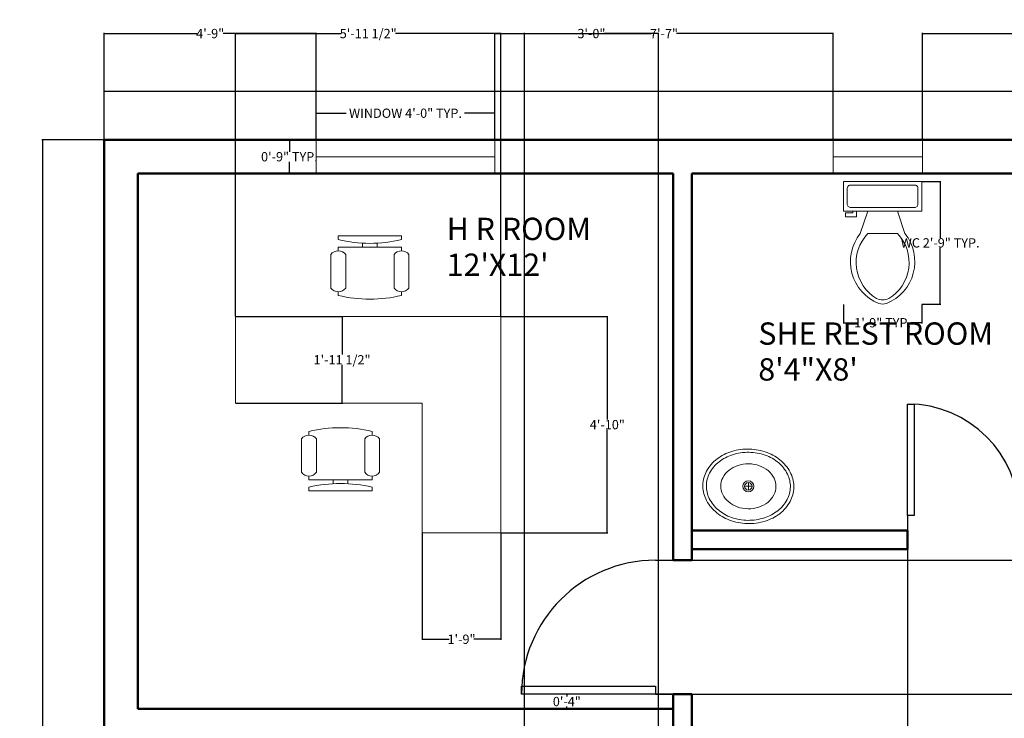
# Model space of a CAD drawing. Units: inches. Extents: x 9441 to 10027, y 18319 to 18830.
# Tile 2 of 4: x 9451 to 9716, y 18642 to 18830. Entities that reach past the tile are written whole.
import ezdxf

# ---------------------------------------------------------------- set-up
doc = ezdxf.new("R2010")
doc.units = ezdxf.units.IN
doc.header["$MEASUREMENT"] = 0
for name, color, linetype, lineweight in [('A-ANNO-DIMS', 2, 'Continuous', 18), ('A-AREA-IDEN', 7, 'Continuous', 25), ('A-DOOR', 3, 'Continuous', 25), ('A-FLOR-FIXT', 9, 'Continuous', 18), ('A-GLAZ', 4, 'Continuous', 18), ('A-WALL', 7, 'Continuous', 50), ('furniture', 8, 'Continuous', 18)]:
    doc.layers.add(name, color=color, linetype=linetype, lineweight=lineweight)
doc.styles.get("Standard").update_dxf_attribs({"font": 'arial.ttf'})
doc.dimstyles.get("Standard").update_dxf_attribs({"dimtxt": 2.5, "dimasz": 0.18, "dimexe": 0.18, "dimexo": 0.0625, "dimgap": 0.09, "dimtad": 0, "dimtih": 1, "dimtoh": 1, "dimdec": 1, "dimzin": 0, "dimdsep": 46, "dimlunit": 3, "dimtxsty": 'Standard', "dimcen": 0.09, "dimadec": 0, "dimazin": 0, "dimtfac": 1, "dimtdec": 1, "dimtofl": 0, "dimtmove": 0, "dimatfit": 3, "dimfxl": 1, "dimtolj": 1, "dimtzin": 0, "dimarcsym": 0})

# ---------------------------------------------------------------- blocks, each defined once
blk = doc.blocks.new('*U2')
for p, q in [((0, 0), (0, -100)), ((750, 0), (750, -100))]:
    blk.add_line(p, q)
blk.add_lwpolyline([(0, 0), (0, 750), (43.75, 750), (43.75, 0)], close=True)
blk.add_arc((0, 0), 750, 0, 90)
blk = doc.blocks.new('*U4')
for p, q in [((0, 100), (0, 0)), ((900, 100), (900, 0)), ((0, 50), (900, 50))]:
    blk.add_line(p, q)
blk = doc.blocks.new('Chair - Desk')
for p, q in [((-8.5, 0), (-8.5, -1)), ((-8.5, 0), (8.5, 0)), ((8.5, 0), (8.5, -1)), ((-2, -3), (-2, -1.9355)), ((2, -1.9576), (2, -3)), ((-10.5, -5), (-10.5, -14)), ((-8.5, -3), (-8.5, -4)), ((-8.5, -3), (8.5, -3)), ((-6.5, -14), (-6.5, -5)), ((6.5, -5), (6.5, -14)), ((8.5, -3), (8.5, -4)), ((10.5, -14), (10.5, -5)), ((-8.5, -15), (-8.5, -16)), ((8.5, -15), (8.5, -16))]:
    blk.add_line(p, q)
for centre, radius, start, end in [((0, 34.625), 36.625, 256.5803, 283.4197), ((-8.5, -6.5), 2.5, 36.8699, 143.1301), ((8.5, -6.5), 2.5, 36.8699, 143.1301), ((-8.5, -12.5), 2.5, 216.8699, 323.1301), ((8.5, -12.5), 2.5, 216.8699, 323.1301), ((0, 19.625), 36.625, 256.5803, 283.4197)]:
    blk.add_arc(centre, radius, start, end)
blk = doc.blocks.new('Toilet - top')
for p, q in [((9.5, -6), (9.5, -2)), ((-10, -8.5), (-8, -8.5)), ((-10, -9.5), (-10, -8.5)), ((-7, -9.5), (-10, -9.5)), ((-8, -8.5), (-8, -8)), ((-7, -8), (-7, -9.5)), ((-4, -8), (-6, -14)), ((4, -8), (6, -14)), ((4, -14), (-4, -14))]:
    blk.add_line(p, q)
blk.add_lwpolyline([(10.5, -8), (10.5, 0), (-10.5, 0), (-10.5, -8)], close=True)
for points in [[(-9.5, -2), (-9.5, -6)], [(8.5, -1), (-8.5, -1)], [(-8.5, -7), (8.5, -7)]]:
    blk.add_lwpolyline(points)
for centre, radius, start, end in [((-8.62, -1.88), 0.884, 81.8699, 188.1301), ((8.62, -1.88), 0.884, 351.8699, 98.1301), ((-8.62, -6.12), 0.884, 171.8699, 278.1301), ((8.62, -6.12), 0.884, 261.8699, 8.1301), ((3.52, -21.58), 12.17, 141.4691, 247.9714), ((4.2, -21.82), 11.33, 136.3677, 238.9468), ((-3.52, -21.58), 12.17, 292.0284, 38.5307), ((-4.2, -21.82), 11.33, 301.053, 43.6321), ((0, -27.88), 4, 245.7318, 294.2682), ((0, -29), 4, 254.8605, 285.1395)]:
    blk.add_arc(centre, radius, start, end)
blk = doc.blocks.new('Sink - Oval top')
for p, q in [((-1, 0), (1, 0)), ((0, 1), (0, -1))]:
    blk.add_line(p, q)
for points in [[(-12.23, 0.39, 0.117634), (-11.46, -3.36, 0.104469), (-8.88, -6.8, 0.090016), (-5.08, -9.07, 0.08192), (-0.32, -10.02, 0.08192), (4.49, -9.38, 0.090016), (8.42, -7.36, 0.104469), (11.22, -4.09, 0.117634), (12.23, -0.39, 0.117634), (11.46, 3.36, 0.104469), (8.88, 6.8, 0.090016), (5.08, 9.07, 0.08192), (0.32, 10.02, 0.08192), (-4.49, 9.38, 0.090016), (-8.42, 7.36, 0.104469), (-11.22, 4.09, 0.117634)], [(-11.29, 0.16, 0.118622), (-10.52, -3.25, 0.104678), (-8.07, -6.36, 0.089562), (-4.54, -8.37, 0.081185), (-0.13, -9.15, 0.081185), (4.3, -8.49, 0.089562), (7.89, -6.58, 0.104678), (10.42, -3.55, 0.118622), (11.29, -0.16, 0.118622), (10.52, 3.25, 0.104678), (8.07, 6.36, 0.089562), (4.54, 8.37, 0.081185), (0.13, 9.15, 0.081185), (-4.3, 8.49, 0.089562), (-7.89, 6.58, 0.104678), (-10.42, 3.55, 0.118622)], [(-7.42, 0.08, 0.118283), (-6.91, -2.17, 0.104607), (-5.29, -4.21, 0.089718), (-2.97, -5.53, 0.081436), (-0.07, -6.04, 0.081436), (2.84, -5.59, 0.089718), (5.2, -4.33, 0.104607), (6.86, -2.32, 0.118283), (7.42, -0.08, 0.118283), (6.91, 2.17, 0.104607), (5.29, 4.21, 0.089718), (2.97, 5.53, 0.081436), (0.07, 6.04, 0.081436), (-2.84, 5.59, 0.089718), (-5.2, 4.33, 0.104607), (-6.86, 2.32, 0.118283)]]:
    blk.add_lwpolyline(points, format="xyb", close=True)
for radius in [1.5, 1]:
    blk.add_circle((0, 0), radius)
blk = doc.blocks.new('*D15')
at = {"layer": 'A-ANNO-DIMS', "color": 0, "lineweight": -2, "transparency": 16777216}
for p, q in [((9473.83, 18797.93), (9457.13, 18797.93)), ((9457.31, 18797.75), (9457.31, 18575.29)), ((9457.31, 18350.11), (9457.31, 18572.56)), ((9473.83, 18349.93), (9457.13, 18349.93))]:
    blk.add_line(p, q, dxfattribs=at)
at = {"layer": 'A-ANNO-DIMS', "color": 0, "transparency": 16777216}
for points in [[(9457.28, 18797.75), (9457.34, 18797.75), (9457.31, 18797.93)], [(9457.28, 18350.11), (9457.34, 18350.11), (9457.31, 18349.93)]]:
    blk.add_solid(points, dxfattribs=at)
at = {"layer": 'Defpoints', "color": 0, "transparency": 16777216}
for p in [(9473.89, 18797.93), (9457.31, 18349.93), (9473.89, 18349.93)]:
    blk.add_point(p, dxfattribs=at)
at = {"layer": 'A-ANNO-DIMS', "color": 0, "transparency": 16777216, "insert": (9457.31, 18573.93), "char_height": 2.5, "attachment_point": 5}
blk.add_mtext('\\A1;37\'-4.0"', dxfattribs=at)
blk = doc.blocks.new('*D16')
at = {"layer": 'A-ANNO-DIMS', "color": 0, "lineweight": -2, "transparency": 16777216}
for p, q in [((9473.89, 18797.99), (9473.89, 18811.27)), ((9474.07, 18811.09), (9728.5, 18811.09)), ((9994.71, 18811.09), (9740.28, 18811.09)), ((9994.89, 18797.99), (9994.89, 18811.27))]:
    blk.add_line(p, q, dxfattribs=at)
at = {"layer": 'A-ANNO-DIMS', "color": 0, "transparency": 16777216}
for points in [[(9474.07, 18811.12), (9474.07, 18811.06), (9473.89, 18811.09)], [(9994.71, 18811.12), (9994.71, 18811.06), (9994.89, 18811.09)]]:
    blk.add_solid(points, dxfattribs=at)
at = {"layer": 'Defpoints', "color": 0, "transparency": 16777216}
for p in [(9994.89, 18811.09), (9473.89, 18797.93), (9994.89, 18797.93)]:
    blk.add_point(p, dxfattribs=at)
at = {"layer": 'A-ANNO-DIMS', "color": 0, "transparency": 16777216, "insert": (9734.39, 18811.09), "char_height": 2.5, "attachment_point": 5}
blk.add_mtext('\\A1;43\'-5.0"', dxfattribs=at)
blk = doc.blocks.new('WIN-FRAME-48x9')
for p, q in [((48, 9), (0, 9)), ((0, 9), (0, 0)), ((48, 0), (48, 9))]:
    blk.add_line(p, q)
blk = doc.blocks.new('WIN-FRAME-24x9')
for p, q in [((0, 0), (0, 9)), ((0, 9), (24, 9)), ((24, 9), (24, 0))]:
    blk.add_line(p, q)
blk = doc.blocks.new('*D23')
at = {"layer": 'A-ANNO-DIMS', "color": 0, "lineweight": -2, "transparency": 16777216}
for p, q in [((9530.89, 18797.99), (9530.89, 18805.31)), ((9531.07, 18805.13), (9538.98, 18805.13)), ((9578.71, 18805.13), (9570.8, 18805.13)), ((9578.89, 18797.99), (9578.89, 18805.31))]:
    blk.add_line(p, q, dxfattribs=at)
at = {"layer": 'A-ANNO-DIMS', "color": 0, "transparency": 16777216}
for points in [[(9531.07, 18805.16), (9531.07, 18805.1), (9530.89, 18805.13)], [(9578.71, 18805.16), (9578.71, 18805.1), (9578.89, 18805.13)]]:
    blk.add_solid(points, dxfattribs=at)
at = {"layer": 'Defpoints', "color": 0, "transparency": 16777216}
for p in [(9578.89, 18805.13), (9530.89, 18797.93), (9578.89, 18797.93)]:
    blk.add_point(p, dxfattribs=at)
at = {"layer": 'A-ANNO-DIMS', "color": 0, "transparency": 16777216, "insert": (9554.89, 18805.13), "char_height": 2.5, "attachment_point": 5}
blk.add_mtext('\\A1;WINDOW 4\'-0" TYP.', dxfattribs=at)
blk = doc.blocks.new('*D24')
at = {"layer": 'A-ANNO-DIMS', "color": 0, "lineweight": -2, "transparency": 16777216}
for p, q in [((9530.83, 18797.93), (9523.51, 18797.93)), ((9523.69, 18797.75), (9523.69, 18794.79)), ((9523.69, 18789.11), (9523.69, 18792.06)), ((9530.83, 18788.93), (9523.51, 18788.93))]:
    blk.add_line(p, q, dxfattribs=at)
at = {"layer": 'A-ANNO-DIMS', "color": 0, "transparency": 16777216}
for points in [[(9523.66, 18797.75), (9523.72, 18797.75), (9523.69, 18797.93)], [(9523.66, 18789.11), (9523.72, 18789.11), (9523.69, 18788.93)]]:
    blk.add_solid(points, dxfattribs=at)
at = {"layer": 'Defpoints', "color": 0, "transparency": 16777216}
for p in [(9523.69, 18797.93), (9530.89, 18797.93), (9530.89, 18788.93)]:
    blk.add_point(p, dxfattribs=at)
at = {"layer": 'A-ANNO-DIMS', "color": 0, "transparency": 16777216, "insert": (9523.69, 18793.43), "char_height": 2.5, "attachment_point": 5}
blk.add_mtext('\\A1;0\'-9" TYP.', dxfattribs=at)
blk = doc.blocks.new('*D25')
at = {"layer": 'A-ANNO-DIMS', "color": 0, "lineweight": -2, "transparency": 16777216}
for p, q in [((9693.75, 18786.8), (9698.82, 18786.8)), ((9698.64, 18786.62), (9698.64, 18771.66)), ((9698.64, 18753.93), (9698.64, 18768.89)), ((9693.75, 18753.75), (9698.82, 18753.75))]:
    blk.add_line(p, q, dxfattribs=at)
at = {"layer": 'A-ANNO-DIMS', "color": 0, "transparency": 16777216}
for points in [[(9698.61, 18786.62), (9698.67, 18786.62), (9698.64, 18786.8)], [(9698.61, 18753.93), (9698.67, 18753.93), (9698.64, 18753.75)]]:
    blk.add_solid(points, dxfattribs=at)
at = {"layer": 'Defpoints', "color": 0, "transparency": 16777216}
for p in [(9693.68, 18786.8), (9698.64, 18786.8), (9693.68, 18753.75)]:
    blk.add_point(p, dxfattribs=at)
at = {"layer": 'A-ANNO-DIMS', "color": 0, "transparency": 16777216, "insert": (9698.64, 18770.27), "char_height": 2.5, "attachment_point": 5}
blk.add_mtext('\\A1;WC 2\'-9" TYP.', dxfattribs=at)
blk = doc.blocks.new('*D26')
at = {"layer": 'A-ANNO-DIMS', "color": 0, "lineweight": -2, "transparency": 16777216}
for p, q in [((9672.68, 18753.69), (9672.68, 18748.61)), ((9693.68, 18753.69), (9693.68, 18748.61)), ((9672.86, 18748.79), (9675.59, 18748.79)), ((9693.5, 18748.79), (9690.78, 18748.79))]:
    blk.add_line(p, q, dxfattribs=at)
at = {"layer": 'A-ANNO-DIMS', "color": 0, "transparency": 16777216}
for points in [[(9672.86, 18748.82), (9672.86, 18748.76), (9672.68, 18748.79)], [(9693.5, 18748.82), (9693.5, 18748.76), (9693.68, 18748.79)]]:
    blk.add_solid(points, dxfattribs=at)
at = {"layer": 'Defpoints', "color": 0, "transparency": 16777216}
for p in [(9672.68, 18753.75), (9693.68, 18753.75), (9693.68, 18748.79)]:
    blk.add_point(p, dxfattribs=at)
at = {"layer": 'A-ANNO-DIMS', "color": 0, "transparency": 16777216, "insert": (9683.18, 18748.79), "char_height": 2.5, "attachment_point": 5}
blk.add_mtext('\\A1;1\'-9" TYP.', dxfattribs=at)
blk = doc.blocks.new('*D41')
at = {"layer": 'A-ANNO-DIMS', "color": 0, "lineweight": -2, "transparency": 16777216}
for p, q in [((9473.89, 18797.99), (9473.89, 18826.73)), ((9474.07, 18826.55), (9498.93, 18826.55)), ((9530.71, 18826.55), (9505.85, 18826.55)), ((9530.89, 18797.99), (9530.89, 18826.73))]:
    blk.add_line(p, q, dxfattribs=at)
at = {"layer": 'A-ANNO-DIMS', "color": 0, "transparency": 16777216}
for points in [[(9474.07, 18826.58), (9474.07, 18826.52), (9473.89, 18826.55)], [(9530.71, 18826.58), (9530.71, 18826.52), (9530.89, 18826.55)]]:
    blk.add_solid(points, dxfattribs=at)
at = {"layer": 'Defpoints', "color": 0, "transparency": 16777216}
for p in [(9530.89, 18826.55), (9473.89, 18797.93), (9530.89, 18797.93)]:
    blk.add_point(p, dxfattribs=at)
at = {"layer": 'A-ANNO-DIMS', "color": 0, "transparency": 16777216, "insert": (9502.39, 18826.55), "char_height": 2.5, "attachment_point": 5}
blk.add_mtext('\\A1;4\'-9"', dxfattribs=at)
blk = doc.blocks.new('*D42')
at = {"layer": 'A-ANNO-DIMS', "color": 0, "lineweight": -2, "transparency": 16777216}
for p, q in [((9578.89, 18797.99), (9578.89, 18826.73)), ((9579.07, 18826.55), (9620.99, 18826.55)), ((9669.71, 18826.55), (9627.79, 18826.55)), ((9669.89, 18797.99), (9669.89, 18826.73))]:
    blk.add_line(p, q, dxfattribs=at)
at = {"layer": 'A-ANNO-DIMS', "color": 0, "transparency": 16777216}
for points in [[(9579.07, 18826.58), (9579.07, 18826.52), (9578.89, 18826.55)], [(9669.71, 18826.58), (9669.71, 18826.52), (9669.89, 18826.55)]]:
    blk.add_solid(points, dxfattribs=at)
at = {"layer": 'Defpoints', "color": 0, "transparency": 16777216}
for p in [(9669.89, 18826.55), (9578.89, 18797.93), (9669.89, 18797.93)]:
    blk.add_point(p, dxfattribs=at)
at = {"layer": 'A-ANNO-DIMS', "color": 0, "transparency": 16777216, "insert": (9624.39, 18826.55), "char_height": 2.5, "attachment_point": 5}
blk.add_mtext('\\A1;7\'-7"', dxfattribs=at)
blk = doc.blocks.new('*D43')
at = {"layer": 'A-ANNO-DIMS', "color": 0, "lineweight": -2, "transparency": 16777216}
for p, q in [((9693.89, 18797.99), (9693.89, 18826.73)), ((9694.07, 18826.55), (9730.97, 18826.55)), ((9774.71, 18826.55), (9737.81, 18826.55)), ((9774.89, 18797.99), (9774.89, 18826.73))]:
    blk.add_line(p, q, dxfattribs=at)
at = {"layer": 'A-ANNO-DIMS', "color": 0, "transparency": 16777216}
for points in [[(9694.07, 18826.58), (9694.07, 18826.52), (9693.89, 18826.55)], [(9774.71, 18826.58), (9774.71, 18826.52), (9774.89, 18826.55)]]:
    blk.add_solid(points, dxfattribs=at)
at = {"layer": 'Defpoints', "color": 0, "transparency": 16777216}
for p in [(9774.89, 18826.55), (9693.89, 18797.93), (9774.89, 18797.93)]:
    blk.add_point(p, dxfattribs=at)
at = {"layer": 'A-ANNO-DIMS', "color": 0, "transparency": 16777216, "insert": (9734.39, 18826.55), "char_height": 2.5, "attachment_point": 5}
blk.add_mtext('\\A1;6\'-9"', dxfattribs=at)
blk = doc.blocks.new('*D47')
at = {"layer": 'A-ANNO-DIMS', "color": 0, "lineweight": -2, "transparency": 16777216}
for p, q in [((9689.89, 18687.86), (9689.89, 18320.95)), ((9719.89, 18687.86), (9719.89, 18320.95)), ((9690.07, 18321.13), (9701.46, 18321.13)), ((9719.71, 18321.13), (9708.32, 18321.13))]:
    blk.add_line(p, q, dxfattribs=at)
at = {"layer": 'A-ANNO-DIMS', "color": 0, "transparency": 16777216}
for points in [[(9690.07, 18321.16), (9690.07, 18321.1), (9689.89, 18321.13)], [(9719.71, 18321.16), (9719.71, 18321.1), (9719.89, 18321.13)]]:
    blk.add_solid(points, dxfattribs=at)
at = {"layer": 'Defpoints', "color": 0, "transparency": 16777216}
for p in [(9689.89, 18687.93), (9719.89, 18687.93), (9719.89, 18321.13)]:
    blk.add_point(p, dxfattribs=at)
at = {"layer": 'A-ANNO-DIMS', "color": 0, "transparency": 16777216, "insert": (9704.89, 18321.13), "char_height": 2.5, "attachment_point": 5}
blk.add_mtext('\\A1;2\'-6"', dxfattribs=at)
blk = doc.blocks.new('*D51')
at = {"layer": 'A-ANNO-DIMS', "color": 0, "lineweight": -2, "transparency": 16777216}
for p, q in [((9631.95, 18684.93), (10023.7, 18684.93)), ((10023.52, 18684.75), (10023.52, 18668.29)), ((10023.52, 18649.11), (10023.52, 18665.56)), ((9631.95, 18648.93), (10023.7, 18648.93))]:
    blk.add_line(p, q, dxfattribs=at)
at = {"layer": 'A-ANNO-DIMS', "color": 0, "transparency": 16777216}
for points in [[(10023.49, 18684.75), (10023.55, 18684.75), (10023.52, 18684.93)], [(10023.49, 18649.11), (10023.55, 18649.11), (10023.52, 18648.93)]]:
    blk.add_solid(points, dxfattribs=at)
at = {"layer": 'Defpoints', "color": 0, "transparency": 16777216}
for p in [(9631.89, 18684.93), (10023.52, 18684.93), (9631.89, 18648.93)]:
    blk.add_point(p, dxfattribs=at)
at = {"layer": 'A-ANNO-DIMS', "color": 0, "transparency": 16777216, "insert": (10023.52, 18666.93), "char_height": 2.5, "attachment_point": 5}
blk.add_mtext('\\A1;3\'-0"', dxfattribs=at)
blk = doc.blocks.new('*D55')
at = {"layer": 'A-ANNO-DIMS', "color": 0, "lineweight": -2, "transparency": 16777216}
for p, q in [((9586.89, 18503.99), (9586.89, 18826.73)), ((9587.07, 18826.55), (9601.48, 18826.55)), ((9622.71, 18826.55), (9608.3, 18826.55)), ((9622.89, 18503.99), (9622.89, 18826.73))]:
    blk.add_line(p, q, dxfattribs=at)
at = {"layer": 'A-ANNO-DIMS', "color": 0, "transparency": 16777216}
for points in [[(9587.07, 18826.58), (9587.07, 18826.52), (9586.89, 18826.55)], [(9622.71, 18826.58), (9622.71, 18826.52), (9622.89, 18826.55)]]:
    blk.add_solid(points, dxfattribs=at)
at = {"layer": 'Defpoints', "color": 0, "transparency": 16777216}
for p in [(9622.89, 18826.55), (9586.89, 18503.93), (9622.89, 18503.93)]:
    blk.add_point(p, dxfattribs=at)
at = {"layer": 'A-ANNO-DIMS', "color": 0, "transparency": 16777216, "insert": (9604.89, 18826.55), "char_height": 2.5, "attachment_point": 5}
blk.add_mtext('\\A1;3\'-0"', dxfattribs=at)
blk = doc.blocks.new('*D64')
at = {"layer": 'A-ANNO-DIMS', "color": 0, "lineweight": -2, "transparency": 16777216}
for p, q in [((9509.22, 18750.54), (9509.22, 18826.73)), ((9509.4, 18826.55), (9537.58, 18826.55)), ((9580.35, 18826.55), (9552.17, 18826.55)), ((9580.53, 18750.54), (9580.53, 18826.73))]:
    blk.add_line(p, q, dxfattribs=at)
at = {"layer": 'A-ANNO-DIMS', "color": 0, "transparency": 16777216}
for points in [[(9509.4, 18826.58), (9509.4, 18826.52), (9509.22, 18826.55)], [(9580.35, 18826.58), (9580.35, 18826.52), (9580.53, 18826.55)]]:
    blk.add_solid(points, dxfattribs=at)
at = {"layer": 'Defpoints', "color": 0, "transparency": 16777216}
for p in [(9580.53, 18826.55), (9509.22, 18750.48), (9580.53, 18750.48)]:
    blk.add_point(p, dxfattribs=at)
at = {"layer": 'A-ANNO-DIMS', "color": 0, "transparency": 16777216, "insert": (9544.87, 18826.55), "char_height": 2.5, "attachment_point": 5}
blk.add_mtext('\\A1;5\'-11 1/2"', dxfattribs=at)
blk = doc.blocks.new('*D65')
at = {"layer": 'A-ANNO-DIMS', "color": 0, "lineweight": -2, "transparency": 16777216}
for p, q in [((9580.6, 18750.48), (9609.34, 18750.48)), ((9609.16, 18750.3), (9609.16, 18722.76)), ((9609.16, 18692.49), (9609.16, 18720.03)), ((9580.6, 18692.31), (9609.34, 18692.31))]:
    blk.add_line(p, q, dxfattribs=at)
at = {"layer": 'A-ANNO-DIMS', "color": 0, "transparency": 16777216}
for points in [[(9609.13, 18750.3), (9609.19, 18750.3), (9609.16, 18750.48)], [(9609.13, 18692.49), (9609.19, 18692.49), (9609.16, 18692.31)]]:
    blk.add_solid(points, dxfattribs=at)
at = {"layer": 'Defpoints', "color": 0, "transparency": 16777216}
for p in [(9580.53, 18750.48), (9580.53, 18692.31), (9609.16, 18692.31)]:
    blk.add_point(p, dxfattribs=at)
at = {"layer": 'A-ANNO-DIMS', "color": 0, "transparency": 16777216, "insert": (9609.16, 18721.39), "char_height": 2.5, "attachment_point": 5}
blk.add_mtext('\\A1;4\'-10"', dxfattribs=at)
blk = doc.blocks.new('*D66')
at = {"layer": 'A-ANNO-DIMS', "color": 0, "lineweight": -2, "transparency": 16777216}
for p, q in [((9509.278343, 18750.479105), (9538.020843, 18750.479105)), ((9537.840843, 18750.299105), (9537.840843, 18740.211121)), ((9537.840843, 18727.357871), (9537.840843, 18737.445855)), ((9509.278343, 18727.177871), (9538.020843, 18727.177871))]:
    blk.add_line(p, q, dxfattribs=at)
at = {"layer": 'A-ANNO-DIMS', "color": 0, "transparency": 16777216}
for points in [[(9537.810843, 18750.299105), (9537.870843, 18750.299105), (9537.840843, 18750.479105)], [(9537.810843, 18727.357871), (9537.870843, 18727.357871), (9537.840843, 18727.177871)]]:
    blk.add_solid(points, dxfattribs=at)
at = {"layer": 'Defpoints', "color": 0, "transparency": 16777216}
for p in [(9509.215843, 18750.479105), (9509.215843, 18727.177871), (9537.840843, 18727.177871)]:
    blk.add_point(p, dxfattribs=at)
at = {"layer": 'A-ANNO-DIMS', "color": 0, "transparency": 16777216, "insert": (9537.840843, 18738.828488), "char_height": 2.5, "attachment_point": 5}
blk.add_mtext('\\A1;1\'-11 1/2"', dxfattribs=at)
blk = doc.blocks.new('*D67')
at = {"layer": 'A-ANNO-DIMS', "color": 0, "lineweight": -2, "transparency": 16777216}
for p, q in [((9559.38, 18692.24), (9559.38, 18663.5)), ((9580.53, 18692.24), (9580.53, 18663.5)), ((9559.56, 18663.68), (9566.66, 18663.68)), ((9580.35, 18663.68), (9573.25, 18663.68))]:
    blk.add_line(p, q, dxfattribs=at)
at = {"layer": 'A-ANNO-DIMS', "color": 0, "transparency": 16777216}
for points in [[(9559.56, 18663.71), (9559.56, 18663.65), (9559.38, 18663.68)], [(9580.35, 18663.71), (9580.35, 18663.65), (9580.53, 18663.68)]]:
    blk.add_solid(points, dxfattribs=at)
at = {"layer": 'Defpoints', "color": 0, "transparency": 16777216}
for p in [(9559.38, 18692.31), (9580.53, 18692.31), (9559.38, 18663.68)]:
    blk.add_point(p, dxfattribs=at)
at = {"layer": 'A-ANNO-DIMS', "color": 0, "transparency": 16777216, "insert": (9569.96, 18663.68), "char_height": 2.5, "attachment_point": 5}
blk.add_mtext('\\A1;1\'-9"', dxfattribs=at)
blk = doc.blocks.new('*D70')
at = {"layer": 'A-ANNO-DIMS', "color": 0, "lineweight": -2, "transparency": 16777216}
for p, q in [((9626.83, 18648.93), (9598.09, 18648.93)), ((9598.27, 18648.75), (9598.27, 18648.29)), ((9626.83, 18644.93), (9598.09, 18644.93)), ((9598.27, 18645.11), (9598.27, 18645.56))]:
    blk.add_line(p, q, dxfattribs=at)
at = {"layer": 'A-ANNO-DIMS', "color": 0, "transparency": 16777216}
for points in [[(9598.24, 18648.75), (9598.3, 18648.75), (9598.27, 18648.93)], [(9598.24, 18645.11), (9598.3, 18645.11), (9598.27, 18644.93)]]:
    blk.add_solid(points, dxfattribs=at)
at = {"layer": 'Defpoints', "color": 0, "transparency": 16777216}
for p in [(9598.27, 18648.93), (9626.89, 18648.93), (9626.89, 18644.93)]:
    blk.add_point(p, dxfattribs=at)
at = {"layer": 'A-ANNO-DIMS', "color": 0, "transparency": 16777216, "insert": (9598.27, 18646.93), "char_height": 2.5, "attachment_point": 5}
blk.add_mtext('\\A1;0\'-4"', dxfattribs=at)

msp = doc.modelspace()

# ---------------------------------------------------------------- linework, layer by layer
at = {"layer": 'A-WALL'}
for p, q in [((9473.89, 18797.93), (9994.89, 18797.93)), ((9473.89, 18797.93), (9473.89, 18349.93)), ((9482.89, 18788.93), (9626.89, 18788.93)), ((9482.89, 18788.93), (9482.89, 18644.93)), ((9626.89, 18684.93), (9626.89, 18788.93)), ((9631.89, 18684.93), (9631.89, 18788.93)), ((9631.89, 18788.93), (9731.89, 18788.93)), ((9631.89, 18692.93), (9689.89, 18692.93)), ((9689.89, 18687.93), (9689.89, 18692.93)), ((9631.89, 18687.93), (9689.89, 18687.93)), ((9631.89, 18684.93), (9626.89, 18684.93)), ((9626.89, 18639.93), (9626.89, 18648.93)), ((9626.89, 18648.93), (9631.89, 18648.93)), ((9631.89, 18639.93), (9631.89, 18648.93)), ((9482.89, 18644.93), (9626.89, 18644.93))]:
    msp.add_line(p, q, dxfattribs=at)
at = {"layer": 'furniture'}
for points in [[(9559.38, 18727.18), (9509.22, 18727.18), (9509.22, 18750.48), (9580.53, 18750.48), (9580.53, 18692.31)], [(9559.38, 18727.18), (9559.38, 18692.31), (9580.53, 18692.31)]]:
    msp.add_lwpolyline(points, dxfattribs=at)

# ---------------------------------------------------------------- block references
at = {"layer": 'A-DOOR', "xscale": 0.0400000000000005, "yscale": 0.0400000000000005, "zscale": 0.0400000000000005}
msp.add_blockref('*U2', (9689.89, 18696.93), dxfattribs=at)
at = {"layer": 'A-DOOR', "xscale": 0.0480000000000006, "yscale": 0.0480000000000006, "zscale": 0.0480000000000006, "rotation": 90}
msp.add_blockref('*U2', (9622.09, 18648.93), dxfattribs=at)
at = {"layer": 'A-FLOR-FIXT'}
for name, p in [('Toilet - top', (9683.18, 18786.8)), ('Sink - Oval top', (9647.08, 18704.81))]:
    msp.add_blockref(name, p, dxfattribs=at)
at = {"layer": 'A-GLAZ'}
for name, p in [('WIN-FRAME-48x9', (9530.89, 18788.93)), ('WIN-FRAME-24x9', (9669.89, 18788.93))]:
    msp.add_blockref(name, p, dxfattribs=at)
for p, xscale, yscale, zscale in [((9530.89, 18790.76), 0.0533333333333332, 0.0533333333333332, 0.0533333333333332), ((9669.89, 18792.09), 0.0266666666666666, 0.0266666666666666, 0.0266666666666666)]:
    msp.add_blockref('*U4', p, dxfattribs=dict(at, xscale=xscale, yscale=yscale, zscale=zscale))
at = {"layer": 'furniture'}
msp.add_blockref('Chair - Desk', (9545.32, 18772.13), dxfattribs=at)
at = {"layer": 'furniture', "rotation": 180}
msp.add_blockref('Chair - Desk', (9537.43, 18703.57), dxfattribs=at)

# ---------------------------------------------------------------- texts
at = {"layer": 'A-AREA-IDEN'}
for s, p in [('H R ROOM', (9565.96, 18771.03)), ("12'X12'", (9565.96, 18761.39)), ('SHE REST ROOM', (9649.75, 18742.88)), ('8\'4"X8\'', (9649.75, 18733.24))]:
    msp.add_text(s, height=6, dxfattribs=at).set_placement(p)

# ---------------------------------------------------------------- dimensions: what is measured, and where the dimension line sits
at = {"layer": 'A-ANNO-DIMS'}
for base, p1, p2, override, picture, middle in [((9580.53, 18826.55), (9509.22, 18750.48), (9580.53, 18750.48), {"dimdec": 1, "dimlfac": 1, "dimrnd": 0, "dimzin": 1, "dimdsep": 46, "dimlunit": 4, "dimfrac": 2}, '*D64', (9544.87, 18826.55)), ((9530.89, 18826.55), (9473.89, 18797.93), (9530.89, 18797.93), {"dimdec": 1, "dimlfac": 1, "dimrnd": 0, "dimzin": 1, "dimdsep": 46, "dimlunit": 4, "dimfrac": 2}, '*D41', (9502.39, 18826.55)), ((9669.89, 18826.55), (9578.89, 18797.93), (9669.89, 18797.93), {"dimdec": 1, "dimlfac": 1, "dimrnd": 0, "dimzin": 1, "dimdsep": 46, "dimlunit": 4, "dimfrac": 2}, '*D42', (9624.39, 18826.55)), ((9622.89, 18826.55), (9586.89, 18503.93), (9622.89, 18503.93), {"dimdec": 1, "dimlfac": 1, "dimrnd": 0, "dimzin": 1, "dimdsep": 46, "dimlunit": 4, "dimfrac": 2}, '*D55', (9604.89, 18826.55)), ((9774.89, 18826.55), (9693.89, 18797.93), (9774.89, 18797.93), {"dimdec": 1, "dimlfac": 1, "dimrnd": 0, "dimzin": 1, "dimdsep": 46, "dimlunit": 4, "dimfrac": 2}, '*D43', (9734.39, 18826.55)), ((9994.89, 18811.09), (9473.89, 18797.93), (9994.89, 18797.93), {"dimclrd": 0, "dimclre": 0, "dimclrt": 0}, '*D16', (9734.39, 18811.09)), ((9719.89, 18321.13), (9689.89, 18687.93), (9719.89, 18687.93), {"dimdec": 1, "dimlfac": 1, "dimrnd": 0, "dimzin": 1, "dimdsep": 46, "dimlunit": 4, "dimfrac": 2}, '*D47', (9704.89, 18321.13))]:
    dim = msp.add_linear_dim(base=base, p1=p1, p2=p2, dimstyle='Standard', override=override, dxfattribs=at)
    dim.commit()
    dim.dimension.update_dxf_attribs({"geometry": picture, "text_midpoint": middle})
for base, p1, p2, text, picture, middle in [((9578.89, 18805.13), (9530.89, 18797.93), (9578.89, 18797.93), 'WINDOW <> TYP.', '*D23', (9554.89, 18805.13)), ((9693.68, 18748.79), (9672.68, 18753.75), (9693.68, 18753.75), '<> TYP.', '*D26', (9683.18, 18748.79))]:
    dim = msp.add_linear_dim(base=base, p1=p1, p2=p2, text=text, dimstyle='Standard', override={"dimdec": 1, "dimlfac": 1, "dimrnd": 0, "dimzin": 1, "dimdsep": 46, "dimlunit": 4, "dimfrac": 2}, dxfattribs=at)
    dim.commit()
    dim.dimension.update_dxf_attribs({"geometry": picture, "text_midpoint": middle})
for base, p1, p2, angle, override, picture, middle in [((9457.31, 18349.93), (9473.89, 18797.93), (9473.89, 18349.93), 90, {"dimclrd": 0, "dimclre": 0, "dimclrt": 0}, '*D15', (9457.31, 18573.93)), ((9537.84, 18727.18), (9509.22, 18750.48), (9509.22, 18727.18), 270, {"dimdec": 1, "dimlfac": 1, "dimrnd": 0, "dimzin": 1, "dimdsep": 46, "dimlunit": 4, "dimfrac": 2}, '*D66', (9537.84, 18738.83)), ((9609.16, 18692.31), (9580.53, 18750.48), (9580.53, 18692.31), 270, {"dimdec": 1, "dimlfac": 1, "dimrnd": 0, "dimzin": 1, "dimdsep": 46, "dimlunit": 4, "dimfrac": 2}, '*D65', (9609.16, 18721.39)), ((9559.3837, 18663.6813), (9580.5331, 18692.3063), (9559.3837, 18692.3063), 180, {"dimdec": 1, "dimlfac": 1, "dimrnd": 0, "dimzin": 1, "dimdsep": 46, "dimlunit": 4, "dimfrac": 2}, '*D67', (9569.9584, 18663.6813)), ((10023.52, 18684.93), (9631.89, 18648.93), (9631.89, 18684.93), 90, {"dimdec": 1, "dimlfac": 1, "dimrnd": 0, "dimzin": 1, "dimdsep": 46, "dimlunit": 4, "dimfrac": 2}, '*D51', (10023.52, 18666.93)), ((9598.27, 18648.93), (9626.89, 18644.93), (9626.89, 18648.93), 90, {"dimdec": 1, "dimlfac": 1, "dimrnd": 0, "dimzin": 1, "dimdsep": 46, "dimlunit": 4, "dimfrac": 2}, '*D70', (9598.27, 18646.93))]:
    dim = msp.add_linear_dim(base=base, p1=p1, p2=p2, angle=angle, dimstyle='Standard', override=override, dxfattribs=at)
    dim.commit()
    dim.dimension.update_dxf_attribs({"geometry": picture, "text_midpoint": middle})
for base, p1, p2, text, picture, middle in [((9523.69, 18797.93), (9530.89, 18788.93), (9530.89, 18797.93), '<> TYP.', '*D24', (9523.69, 18793.43)), ((9698.6416, 18786.796), (9693.6846, 18753.7497), (9693.6846, 18786.796), 'WC <> TYP.', '*D25', (9698.6416, 18770.2728))]:
    dim = msp.add_linear_dim(base=base, p1=p1, p2=p2, angle=90, text=text, dimstyle='Standard', override={"dimdec": 1, "dimlfac": 1, "dimrnd": 0, "dimzin": 1, "dimdsep": 46, "dimlunit": 4, "dimfrac": 2}, dxfattribs=at)
    dim.commit()
    dim.dimension.update_dxf_attribs({"geometry": picture, "text_midpoint": middle})

doc.saveas('drawing.dxf')
